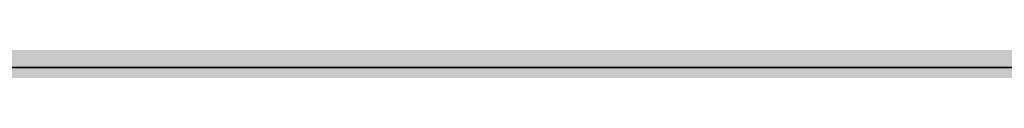
# Model space of a CAD drawing. Units: millimetres. Extents: x -22994 to 29398, y -19990 to 20176.
# Tile 96 of 135: x 229.428 to 230.597, y 84.556 to 84.571. Entities that reach past the tile are written whole.
import ezdxf
from ezdxf import colors
from ezdxf.entities.mleader import LeaderData, LeaderLine
from ezdxf.math import Vec2, Vec3

# ---------------------------------------------------------------- set-up
doc = ezdxf.new("R2010")
doc.units = ezdxf.units.MM
doc.header["$MEASUREMENT"] = 0
for name, color, linetype, lineweight in [('M-ANNO-TEXT', 7, 'Continuous', 25), ('M-DIMS', 2, 'Continuous', 18), ('M-EQPM-PATT', 7, 'Continuous', 18), ('M-PIPE', 7, 'Continuous', 35)]:
    doc.layers.add(name, color=color, linetype=linetype, lineweight=lineweight)
doc.styles.get("Standard").update_dxf_attribs({"font": 'arial.ttf'})
doc.dimstyles.get("Standard").update_dxf_attribs({"dimtxt": 0.18, "dimasz": 10000, "dimexe": 0.18, "dimexo": 0.0625, "dimgap": 0.09, "dimtad": 0, "dimtih": 1, "dimtoh": 1, "dimdec": 0, "dimzin": 0, "dimdsep": 46, "dimtxsty": 'Standard', "dimcen": 0.09, "dimadec": 0, "dimazin": 0, "dimtfac": 1, "dimtdec": 0, "dimtofl": 0, "dimtmove": 0, "dimatfit": 3, "dimfxl": 1, "dimtolj": 1, "dimtzin": 0, "dimlwd": 30, "dimarcsym": 0})

# ---------------------------------------------------------------- blocks, each defined once
blk = doc.blocks.new('*D2')
at = {"layer": 'Defpoints', "color": 0, "transparency": 16777216}
for p in [(6.6773, 10.2713), (290.852, 10.2713), (290.852, -5.0787)]:
    blk.add_point(p, dxfattribs=at)
at = {"layer": 'M-DIMS', "color": 0, "lineweight": -2, "transparency": 16777216}
for p, q in [((6.6773, 10.2088), (6.6773, -5.2587)), ((290.852, 10.2088), (290.852, -5.2587))]:
    blk.add_line(p, q, dxfattribs=at)
at = {"layer": 'M-DIMS', "color": 0, "lineweight": 30, "transparency": 16777216}
for p, q in [((-9993.3227, -5.0787), (-19993.3227, -5.0787)), ((10290.852, -5.0787), (20290.852, -5.0787))]:
    blk.add_line(p, q, dxfattribs=at)
at = {"layer": 'M-DIMS', "color": 0, "transparency": 16777216}
for points in [[(-9993.3227, 1661.5879), (-9993.3227, -1671.7454), (6.6773, -5.0787)], [(10290.852, 1661.5879), (10290.852, -1671.7454), (290.852, -5.0787)]]:
    blk.add_solid(points, dxfattribs=at)
at = {"layer": 'M-DIMS', "color": 0, "transparency": 16777216, "insert": (148.7647, -5.0787), "char_height": 0.18, "attachment_point": 5}
blk.add_mtext('\\A1;284.2', dxfattribs=at)
blk = doc.blocks.new('*D3')
at = {"layer": 'Defpoints', "color": 0, "transparency": 16777216}
for p in [(110.2647, 204.1654), (110.2647, 176.3662), (95.8327, 127.967)]:
    blk.add_point(p, dxfattribs=at)
at = {"layer": 'M-DIMS', "color": 0, "lineweight": -2, "transparency": 16777216}
for p, q in [((95.8327, 128.0295), (95.8327, 204.3454)), ((110.2647, 176.4287), (110.2647, 204.3454))]:
    blk.add_line(p, q, dxfattribs=at)
at = {"layer": 'M-DIMS', "color": 0, "lineweight": 30, "transparency": 16777216}
for p, q in [((-9904.1673, 204.1654), (-19904.1673, 204.1654)), ((10110.2647, 204.1654), (20110.2647, 204.1654))]:
    blk.add_line(p, q, dxfattribs=at)
at = {"layer": 'M-DIMS', "color": 0, "transparency": 16777216}
for points in [[(-9904.1673, 1870.8321), (-9904.1673, -1462.5013), (95.8327, 204.1654)], [(10110.2647, 1870.8321), (10110.2647, -1462.5013), (110.2647, 204.1654)]]:
    blk.add_solid(points, dxfattribs=at)
at = {"layer": 'M-DIMS', "color": 0, "transparency": 16777216, "insert": (103.0487, 204.1654), "char_height": 0.18, "attachment_point": 5}
blk.add_mtext('\\A1;14.432', dxfattribs=at)
blk = doc.blocks.new('*D4')
at = {"layer": 'Defpoints', "color": 0, "transparency": 16777216}
for p in [(116.2647, 204.1654), (110.2647, 176.3662), (116.2647, 176.3662)]:
    blk.add_point(p, dxfattribs=at)
at = {"layer": 'M-DIMS', "color": 0, "lineweight": -2, "transparency": 16777216}
for p, q in [((110.2647, 176.4287), (110.2647, 204.3454)), ((116.2647, 176.4287), (116.2647, 204.3454))]:
    blk.add_line(p, q, dxfattribs=at)
at = {"layer": 'M-DIMS', "color": 0, "lineweight": 30, "transparency": 16777216}
for p, q in [((-9889.7353, 204.1654), (-19889.7353, 204.1654)), ((10116.2647, 204.1654), (20116.2647, 204.1654))]:
    blk.add_line(p, q, dxfattribs=at)
at = {"layer": 'M-DIMS', "color": 0, "transparency": 16777216}
for points in [[(-9889.7353, 1870.8321), (-9889.7353, -1462.5013), (110.2647, 204.1654)], [(10116.2647, 1870.8321), (10116.2647, -1462.5013), (116.2647, 204.1654)]]:
    blk.add_solid(points, dxfattribs=at)
at = {"layer": 'M-DIMS', "color": 0, "transparency": 16777216, "insert": (113.2647, 204.1654), "char_height": 0.18, "attachment_point": 5}
blk.add_mtext('\\A1;6', dxfattribs=at)
blk = doc.blocks.new('*D5')
at = {"layer": 'Defpoints', "color": 0, "transparency": 16777216}
for p in [(181.2647, 204.1654), (116.2647, 176.3662), (181.2647, 176.3662)]:
    blk.add_point(p, dxfattribs=at)
at = {"layer": 'M-DIMS', "color": 0, "lineweight": -2, "transparency": 16777216}
for p, q in [((116.2647, 176.4287), (116.2647, 204.3454)), ((181.2647, 176.4287), (181.2647, 204.3454))]:
    blk.add_line(p, q, dxfattribs=at)
at = {"layer": 'M-DIMS', "color": 0, "lineweight": 30, "transparency": 16777216}
for p, q in [((-9883.7353, 204.1654), (-19883.7353, 204.1654)), ((10181.2647, 204.1654), (20181.2647, 204.1654))]:
    blk.add_line(p, q, dxfattribs=at)
at = {"layer": 'M-DIMS', "color": 0, "transparency": 16777216}
for points in [[(-9883.7353, 1870.8321), (-9883.7353, -1462.5013), (116.2647, 204.1654)], [(10181.2647, 1870.8321), (10181.2647, -1462.5013), (181.2647, 204.1654)]]:
    blk.add_solid(points, dxfattribs=at)
at = {"layer": 'M-DIMS', "color": 0, "transparency": 16777216, "insert": (148.7647, 204.1654), "char_height": 0.18, "attachment_point": 5}
blk.add_mtext('\\A1;65', dxfattribs=at)
blk = doc.blocks.new('*D6')
at = {"layer": 'Defpoints', "color": 0, "transparency": 16777216}
for p in [(187.2647, 204.1654), (181.2647, 176.3662), (187.2647, 176.3662)]:
    blk.add_point(p, dxfattribs=at)
at = {"layer": 'M-DIMS', "color": 0, "lineweight": -2, "transparency": 16777216}
for p, q in [((181.2647, 176.4287), (181.2647, 204.3454)), ((187.2647, 176.4287), (187.2647, 204.3454))]:
    blk.add_line(p, q, dxfattribs=at)
at = {"layer": 'M-DIMS', "color": 0, "lineweight": 30, "transparency": 16777216}
for p, q in [((-9818.7353, 204.1654), (-19818.7353, 204.1654)), ((10187.2647, 204.1654), (20187.2647, 204.1654))]:
    blk.add_line(p, q, dxfattribs=at)
at = {"layer": 'M-DIMS', "color": 0, "transparency": 16777216}
for points in [[(-9818.7353, 1870.8321), (-9818.7353, -1462.5013), (181.2647, 204.1654)], [(10187.2647, 1870.8321), (10187.2647, -1462.5013), (187.2647, 204.1654)]]:
    blk.add_solid(points, dxfattribs=at)
at = {"layer": 'M-DIMS', "color": 0, "transparency": 16777216, "insert": (184.2647, 204.1654), "char_height": 0.18, "attachment_point": 5}
blk.add_mtext('\\A1;6', dxfattribs=at)
blk = doc.blocks.new('*D7')
at = {"layer": 'Defpoints', "color": 0, "transparency": 16777216}
for p in [(201.6967, 204.1654), (187.2647, 176.3662), (201.6967, 127.967)]:
    blk.add_point(p, dxfattribs=at)
at = {"layer": 'M-DIMS', "color": 0, "lineweight": -2, "transparency": 16777216}
for p, q in [((187.2647, 176.4287), (187.2647, 204.3454)), ((201.6967, 128.0295), (201.6967, 204.3454))]:
    blk.add_line(p, q, dxfattribs=at)
at = {"layer": 'M-DIMS', "color": 0, "lineweight": 30, "transparency": 16777216}
for p, q in [((-9812.7353, 204.1654), (-19812.7353, 204.1654)), ((10201.6967, 204.1654), (20201.6967, 204.1654))]:
    blk.add_line(p, q, dxfattribs=at)
at = {"layer": 'M-DIMS', "color": 0, "transparency": 16777216}
for points in [[(-9812.7353, 1870.8321), (-9812.7353, -1462.5013), (187.2647, 204.1654)], [(10201.6967, 1870.8321), (10201.6967, -1462.5013), (201.6967, 204.1654)]]:
    blk.add_solid(points, dxfattribs=at)
at = {"layer": 'M-DIMS', "color": 0, "transparency": 16777216, "insert": (194.4807, 204.1654), "char_height": 0.18, "attachment_point": 5}
blk.add_mtext('\\A1;14.432', dxfattribs=at)
blk = doc.blocks.new('*D8')
at = {"layer": 'Defpoints', "color": 0, "transparency": 16777216}
for p in [(227.6485, 204.1654), (227.6485, 146.7296), (201.6967, 127.967)]:
    blk.add_point(p, dxfattribs=at)
at = {"layer": 'M-DIMS', "color": 0, "lineweight": -2, "transparency": 16777216}
for p, q in [((201.6967, 128.0295), (201.6967, 204.3454)), ((227.6485, 146.7921), (227.6485, 204.3454))]:
    blk.add_line(p, q, dxfattribs=at)
at = {"layer": 'M-DIMS', "color": 0, "lineweight": 30, "transparency": 16777216}
for p, q in [((-9798.3033, 204.1654), (-19798.3033, 204.1654)), ((10227.6485, 204.1654), (20227.6485, 204.1654))]:
    blk.add_line(p, q, dxfattribs=at)
at = {"layer": 'M-DIMS', "color": 0, "transparency": 16777216}
for points in [[(-9798.3033, 1870.8321), (-9798.3033, -1462.5013), (201.6967, 204.1654)], [(10227.6485, 1870.8321), (10227.6485, -1462.5013), (227.6485, 204.1654)]]:
    blk.add_solid(points, dxfattribs=at)
at = {"layer": 'M-DIMS', "color": 0, "transparency": 16777216, "insert": (214.6726, 204.1654), "char_height": 0.18, "attachment_point": 5}
blk.add_mtext('\\A1;25.95', dxfattribs=at)
blk = doc.blocks.new('*D9')
at = {"layer": 'Defpoints', "color": 0, "transparency": 16777216}
for p in [(187.2647, 176.3662), (306.202, 176.3662), (290.852, 10.2713)]:
    blk.add_point(p, dxfattribs=at)
at = {"layer": 'M-DIMS', "color": 0, "lineweight": 30, "transparency": 16777216}
for p, q in [((306.202, 10176.3662), (306.202, 20176.3662)), ((306.202, -9989.7287), (306.202, -19989.7287))]:
    blk.add_line(p, q, dxfattribs=at)
at = {"layer": 'M-DIMS', "color": 0, "lineweight": -2, "transparency": 16777216}
for p, q in [((187.3272, 176.3662), (306.382, 176.3662)), ((290.9145, 10.2713), (306.382, 10.2713))]:
    blk.add_line(p, q, dxfattribs=at)
at = {"layer": 'M-DIMS', "color": 0, "transparency": 16777216}
for points in [[(-1360.4646, 10176.3662), (1972.8687, 10176.3662), (306.202, 176.3662)], [(-1360.4646, -9989.7287), (1972.8687, -9989.7287), (306.202, 10.2713)]]:
    blk.add_solid(points, dxfattribs=at)
at = {"layer": 'M-DIMS', "color": 0, "transparency": 16777216, "insert": (306.202, 93.3187), "char_height": 0.18, "attachment_point": 5}
blk.add_mtext('\\A1;166.1', dxfattribs=at)
blk = doc.blocks.new('*D10')
at = {"layer": 'Defpoints', "color": 0, "transparency": 16777216}
for p in [(125.6498, 136.0713), (133.3459, 136.0713), (133.3459, -5.0787)]:
    blk.add_point(p, dxfattribs=at)
at = {"layer": 'M-DIMS', "color": 0, "lineweight": -2, "transparency": 16777216}
for p, q in [((125.6498, 136.0088), (125.6498, -5.2587)), ((133.3459, 136.0088), (133.3459, -5.2587))]:
    blk.add_line(p, q, dxfattribs=at)
at = {"layer": 'M-DIMS', "color": 0, "lineweight": 30, "transparency": 16777216}
for p, q in [((-9874.3502, -5.0787), (-19874.3502, -5.0787)), ((10133.3459, -5.0787), (20133.3459, -5.0787))]:
    blk.add_line(p, q, dxfattribs=at)
at = {"layer": 'M-DIMS', "color": 0, "transparency": 16777216}
for points in [[(-9874.3502, 1661.5879), (-9874.3502, -1671.7454), (125.6498, -5.0787)], [(10133.3459, 1661.5879), (10133.3459, -1671.7454), (133.3459, -5.0787)]]:
    blk.add_solid(points, dxfattribs=at)
at = {"layer": 'M-DIMS', "color": 0, "transparency": 16777216, "insert": (129.4978, -5.0787), "char_height": 0.18, "attachment_point": 5}
blk.add_mtext('\\A1;7.696', dxfattribs=at)
blk = doc.blocks.new('*D11')
at = {"layer": 'Defpoints', "color": 0, "transparency": 16777216}
for p in [(133.3459, 136.0713), (135.6498, 136.0713), (135.6498, -5.0787)]:
    blk.add_point(p, dxfattribs=at)
at = {"layer": 'M-DIMS', "color": 0, "lineweight": -2, "transparency": 16777216}
for p, q in [((133.3459, 136.0088), (133.3459, -5.2587)), ((135.6498, 136.0088), (135.6498, -5.2587))]:
    blk.add_line(p, q, dxfattribs=at)
at = {"layer": 'M-DIMS', "color": 0, "lineweight": 30, "transparency": 16777216}
for p, q in [((-9866.6541, -5.0787), (-19866.6541, -5.0787)), ((10135.6498, -5.0787), (20135.6498, -5.0787))]:
    blk.add_line(p, q, dxfattribs=at)
at = {"layer": 'M-DIMS', "color": 0, "transparency": 16777216}
for points in [[(-9866.6541, 1661.5879), (-9866.6541, -1671.7454), (133.3459, -5.0787)], [(10135.6498, 1661.5879), (10135.6498, -1671.7454), (135.6498, -5.0787)]]:
    blk.add_solid(points, dxfattribs=at)
at = {"layer": 'M-DIMS', "color": 0, "transparency": 16777216, "insert": (134.4978, -5.0787), "char_height": 0.18, "attachment_point": 5}
blk.add_mtext('\\A1;2.304', dxfattribs=at)
blk = doc.blocks.new('*D12')
at = {"layer": 'Defpoints', "color": 0, "transparency": 16777216}
for p in [(135.6498, 136.0713), (145.6498, 136.0713), (145.6498, -5.0787)]:
    blk.add_point(p, dxfattribs=at)
at = {"layer": 'M-DIMS', "color": 0, "lineweight": -2, "transparency": 16777216}
for p, q in [((135.6498, 136.0088), (135.6498, -5.2587)), ((145.6498, 136.0088), (145.6498, -5.2587))]:
    blk.add_line(p, q, dxfattribs=at)
at = {"layer": 'M-DIMS', "color": 0, "lineweight": 30, "transparency": 16777216}
for p, q in [((-9864.3502, -5.0787), (-19864.3502, -5.0787)), ((10145.6498, -5.0787), (20145.6498, -5.0787))]:
    blk.add_line(p, q, dxfattribs=at)
at = {"layer": 'M-DIMS', "color": 0, "transparency": 16777216}
for points in [[(-9864.3502, 1661.5879), (-9864.3502, -1671.7454), (135.6498, -5.0787)], [(10145.6498, 1661.5879), (10145.6498, -1671.7454), (145.6498, -5.0787)]]:
    blk.add_solid(points, dxfattribs=at)
at = {"layer": 'M-DIMS', "color": 0, "transparency": 16777216, "insert": (140.6498, -5.0787), "char_height": 0.18, "attachment_point": 5}
blk.add_mtext('\\A1;10', dxfattribs=at)
blk = doc.blocks.new('*D13')
at = {"layer": 'Defpoints', "color": 0, "transparency": 16777216}
for p in [(145.6498, 136.0713), (155.6498, 136.0713), (155.6498, -5.0787)]:
    blk.add_point(p, dxfattribs=at)
at = {"layer": 'M-DIMS', "color": 0, "lineweight": -2, "transparency": 16777216}
for p, q in [((145.6498, 136.0088), (145.6498, -5.2587)), ((155.6498, 136.0088), (155.6498, -5.2587))]:
    blk.add_line(p, q, dxfattribs=at)
at = {"layer": 'M-DIMS', "color": 0, "lineweight": 30, "transparency": 16777216}
for p, q in [((-9854.3502, -5.0787), (-19854.3502, -5.0787)), ((10155.6498, -5.0787), (20155.6498, -5.0787))]:
    blk.add_line(p, q, dxfattribs=at)
at = {"layer": 'M-DIMS', "color": 0, "transparency": 16777216}
for points in [[(-9854.3502, 1661.5879), (-9854.3502, -1671.7454), (145.6498, -5.0787)], [(10155.6498, 1661.5879), (10155.6498, -1671.7454), (155.6498, -5.0787)]]:
    blk.add_solid(points, dxfattribs=at)
at = {"layer": 'M-DIMS', "color": 0, "transparency": 16777216, "insert": (150.6498, -5.0787), "char_height": 0.18, "attachment_point": 5}
blk.add_mtext('\\A1;10', dxfattribs=at)
blk = doc.blocks.new('*D14')
at = {"layer": 'Defpoints', "color": 0, "transparency": 16777216}
for p in [(155.6498, 136.0713), (165.6498, 136.0713), (165.6498, -5.0787)]:
    blk.add_point(p, dxfattribs=at)
at = {"layer": 'M-DIMS', "color": 0, "lineweight": -2, "transparency": 16777216}
for p, q in [((155.6498, 136.0088), (155.6498, -5.2587)), ((165.6498, 136.0088), (165.6498, -5.2587))]:
    blk.add_line(p, q, dxfattribs=at)
at = {"layer": 'M-DIMS', "color": 0, "lineweight": 30, "transparency": 16777216}
for p, q in [((-9844.3502, -5.0787), (-19844.3502, -5.0787)), ((10165.6498, -5.0787), (20165.6498, -5.0787))]:
    blk.add_line(p, q, dxfattribs=at)
at = {"layer": 'M-DIMS', "color": 0, "transparency": 16777216}
for points in [[(-9844.3502, 1661.5879), (-9844.3502, -1671.7454), (155.6498, -5.0787)], [(10165.6498, 1661.5879), (10165.6498, -1671.7454), (165.6498, -5.0787)]]:
    blk.add_solid(points, dxfattribs=at)
at = {"layer": 'M-DIMS', "color": 0, "transparency": 16777216, "insert": (160.6498, -5.0787), "char_height": 0.18, "attachment_point": 5}
blk.add_mtext('\\A1;10', dxfattribs=at)
blk = doc.blocks.new('*D15')
at = {"layer": 'Defpoints', "color": 0, "transparency": 16777216}
for p in [(173.3459, 154.788), (173.3459, 136.0713), (306.202, 136.0713)]:
    blk.add_point(p, dxfattribs=at)
at = {"layer": 'M-DIMS', "color": 0, "lineweight": 30, "transparency": 16777216}
for p, q in [((306.202, 10154.788), (306.202, 20154.788)), ((306.202, -9863.9287), (306.202, -19863.9287))]:
    blk.add_line(p, q, dxfattribs=at)
at = {"layer": 'M-DIMS', "color": 0, "lineweight": -2, "transparency": 16777216}
for p, q in [((173.4084, 154.788), (306.382, 154.788)), ((173.4084, 136.0713), (306.382, 136.0713))]:
    blk.add_line(p, q, dxfattribs=at)
at = {"layer": 'M-DIMS', "color": 0, "transparency": 16777216}
for points in [[(-1360.4646, 10154.788), (1972.8687, 10154.788), (306.202, 154.788)], [(-1360.4646, -9863.9287), (1972.8687, -9863.9287), (306.202, 136.0713)]]:
    blk.add_solid(points, dxfattribs=at)
at = {"layer": 'M-DIMS', "color": 0, "transparency": 16777216, "insert": (306.202, 145.4297), "char_height": 0.18, "attachment_point": 5}
blk.add_mtext('\\A1;18.717', dxfattribs=at)
blk = doc.blocks.new('*D16')
at = {"layer": 'Defpoints', "color": 0, "transparency": 16777216}
for p in [(120.1702, 204.1654), (110.4658, 48.0349), (120.1702, 48.0349)]:
    blk.add_point(p, dxfattribs=at)
at = {"layer": 'M-DIMS', "color": 0, "lineweight": -2, "transparency": 16777216}
for p, q in [((110.4658, 48.0974), (110.4658, 204.3454)), ((120.1702, 48.0974), (120.1702, 204.3454))]:
    blk.add_line(p, q, dxfattribs=at)
at = {"layer": 'M-DIMS', "color": 0, "lineweight": 30, "transparency": 16777216}
for p, q in [((-9889.5342, 204.1654), (-19889.5342, 204.1654)), ((10120.1702, 204.1654), (20120.1702, 204.1654))]:
    blk.add_line(p, q, dxfattribs=at)
at = {"layer": 'M-DIMS', "color": 0, "transparency": 16777216}
for points in [[(-9889.5342, 1870.8321), (-9889.5342, -1462.5013), (110.4658, 204.1654)], [(10120.1702, 1870.8321), (10120.1702, -1462.5013), (120.1702, 204.1654)]]:
    blk.add_solid(points, dxfattribs=at)
at = {"layer": 'M-DIMS', "color": 0, "transparency": 16777216, "insert": (115.318, 204.1654), "char_height": 0.18, "attachment_point": 5}
blk.add_mtext('\\A1;9.704', dxfattribs=at)
blk = doc.blocks.new('*D17')
at = {"layer": 'Defpoints', "color": 0, "transparency": 16777216}
for p in [(126.1702, 204.1654), (120.1702, 48.0349), (126.1702, 48.0349)]:
    blk.add_point(p, dxfattribs=at)
at = {"layer": 'M-DIMS', "color": 0, "lineweight": -2, "transparency": 16777216}
for p, q in [((120.1702, 48.0974), (120.1702, 204.3454)), ((126.1702, 48.0974), (126.1702, 204.3454))]:
    blk.add_line(p, q, dxfattribs=at)
at = {"layer": 'M-DIMS', "color": 0, "lineweight": 30, "transparency": 16777216}
for p, q in [((-9879.8298, 204.1654), (-19879.8298, 204.1654)), ((10126.1702, 204.1654), (20126.1702, 204.1654))]:
    blk.add_line(p, q, dxfattribs=at)
at = {"layer": 'M-DIMS', "color": 0, "transparency": 16777216}
for points in [[(-9879.8298, 1870.8321), (-9879.8298, -1462.5013), (120.1702, 204.1654)], [(10126.1702, 1870.8321), (10126.1702, -1462.5013), (126.1702, 204.1654)]]:
    blk.add_solid(points, dxfattribs=at)
at = {"layer": 'M-DIMS', "color": 0, "transparency": 16777216, "insert": (123.1702, 204.1654), "char_height": 0.18, "attachment_point": 5}
blk.add_mtext('\\A1;6', dxfattribs=at)
blk = doc.blocks.new('*D18')
at = {"layer": 'Defpoints', "color": 0, "transparency": 16777216}
for p in [(132.1702, 204.1654), (126.1702, 48.0349), (132.1702, 48.0349)]:
    blk.add_point(p, dxfattribs=at)
at = {"layer": 'M-DIMS', "color": 0, "lineweight": -2, "transparency": 16777216}
for p, q in [((126.1702, 48.0974), (126.1702, 204.3454)), ((132.1702, 48.0974), (132.1702, 204.3454))]:
    blk.add_line(p, q, dxfattribs=at)
at = {"layer": 'M-DIMS', "color": 0, "lineweight": 30, "transparency": 16777216}
for p, q in [((-9873.8298, 204.1654), (-19873.8298, 204.1654)), ((10132.1702, 204.1654), (20132.1702, 204.1654))]:
    blk.add_line(p, q, dxfattribs=at)
at = {"layer": 'M-DIMS', "color": 0, "transparency": 16777216}
for points in [[(-9873.8298, 1870.8321), (-9873.8298, -1462.5013), (126.1702, 204.1654)], [(10132.1702, 1870.8321), (10132.1702, -1462.5013), (132.1702, 204.1654)]]:
    blk.add_solid(points, dxfattribs=at)
at = {"layer": 'M-DIMS', "color": 0, "transparency": 16777216, "insert": (129.1702, 204.1654), "char_height": 0.18, "attachment_point": 5}
blk.add_mtext('\\A1;6', dxfattribs=at)
blk = doc.blocks.new('*D19')
at = {"layer": 'Defpoints', "color": 0, "transparency": 16777216}
for p in [(138.1702, 204.1654), (132.1702, 48.0349), (138.1702, 48.0349)]:
    blk.add_point(p, dxfattribs=at)
at = {"layer": 'M-DIMS', "color": 0, "lineweight": -2, "transparency": 16777216}
for p, q in [((132.1702, 48.0974), (132.1702, 204.3454)), ((138.1702, 48.0974), (138.1702, 204.3454))]:
    blk.add_line(p, q, dxfattribs=at)
at = {"layer": 'M-DIMS', "color": 0, "lineweight": 30, "transparency": 16777216}
for p, q in [((-9867.8298, 204.1654), (-19867.8298, 204.1654)), ((10138.1702, 204.1654), (20138.1702, 204.1654))]:
    blk.add_line(p, q, dxfattribs=at)
at = {"layer": 'M-DIMS', "color": 0, "transparency": 16777216}
for points in [[(-9867.8298, 1870.8321), (-9867.8298, -1462.5013), (132.1702, 204.1654)], [(10138.1702, 1870.8321), (10138.1702, -1462.5013), (138.1702, 204.1654)]]:
    blk.add_solid(points, dxfattribs=at)
at = {"layer": 'M-DIMS', "color": 0, "transparency": 16777216, "insert": (135.1702, 204.1654), "char_height": 0.18, "attachment_point": 5}
blk.add_mtext('\\A1;6', dxfattribs=at)
blk = doc.blocks.new('*D20')
at = {"layer": 'Defpoints', "color": 0, "transparency": 16777216}
for p in [(144.1702, 204.1654), (138.1702, 48.0349), (144.1702, 48.0349)]:
    blk.add_point(p, dxfattribs=at)
at = {"layer": 'M-DIMS', "color": 0, "lineweight": -2, "transparency": 16777216}
for p, q in [((138.1702, 48.0974), (138.1702, 204.3454)), ((144.1702, 48.0974), (144.1702, 204.3454))]:
    blk.add_line(p, q, dxfattribs=at)
at = {"layer": 'M-DIMS', "color": 0, "lineweight": 30, "transparency": 16777216}
for p, q in [((-9861.8298, 204.1654), (-19861.8298, 204.1654)), ((10144.1702, 204.1654), (20144.1702, 204.1654))]:
    blk.add_line(p, q, dxfattribs=at)
at = {"layer": 'M-DIMS', "color": 0, "transparency": 16777216}
for points in [[(-9861.8298, 1870.8321), (-9861.8298, -1462.5013), (138.1702, 204.1654)], [(10144.1702, 1870.8321), (10144.1702, -1462.5013), (144.1702, 204.1654)]]:
    blk.add_solid(points, dxfattribs=at)
at = {"layer": 'M-DIMS', "color": 0, "transparency": 16777216, "insert": (141.1702, 204.1654), "char_height": 0.18, "attachment_point": 5}
blk.add_mtext('\\A1;6', dxfattribs=at)
blk = doc.blocks.new('*D21')
at = {"layer": 'Defpoints', "color": 0, "transparency": 16777216}
for p in [(149.1157, 204.1654), (144.1702, 48.0349), (149.1157, 48.0349)]:
    blk.add_point(p, dxfattribs=at)
at = {"layer": 'M-DIMS', "color": 0, "lineweight": -2, "transparency": 16777216}
for p, q in [((144.1702, 48.0974), (144.1702, 204.3454)), ((149.1157, 48.0974), (149.1157, 204.3454))]:
    blk.add_line(p, q, dxfattribs=at)
at = {"layer": 'M-DIMS', "color": 0, "lineweight": 30, "transparency": 16777216}
for p, q in [((-9855.8298, 204.1654), (-19855.8298, 204.1654)), ((10149.1157, 204.1654), (20149.1157, 204.1654))]:
    blk.add_line(p, q, dxfattribs=at)
at = {"layer": 'M-DIMS', "color": 0, "transparency": 16777216}
for points in [[(-9855.8298, 1870.8321), (-9855.8298, -1462.5013), (144.1702, 204.1654)], [(10149.1157, 1870.8321), (10149.1157, -1462.5013), (149.1157, 204.1654)]]:
    blk.add_solid(points, dxfattribs=at)
at = {"layer": 'M-DIMS', "color": 0, "transparency": 16777216, "insert": (146.6429, 204.1654), "char_height": 0.18, "attachment_point": 5}
blk.add_mtext('\\A1;4.945', dxfattribs=at)
blk = doc.blocks.new('*D22')
at = {"layer": 'Defpoints', "color": 0, "transparency": 16777216}
for p in [(149.1157, 30.9895), (155.1157, 30.9895), (155.1157, -5.0787)]:
    blk.add_point(p, dxfattribs=at)
at = {"layer": 'M-DIMS', "color": 0, "lineweight": -2, "transparency": 16777216}
for p, q in [((149.1157, 30.927), (149.1157, -5.2587)), ((155.1157, 30.927), (155.1157, -5.2587))]:
    blk.add_line(p, q, dxfattribs=at)
at = {"layer": 'M-DIMS', "color": 0, "lineweight": 30, "transparency": 16777216}
for p, q in [((-9850.8843, -5.0787), (-19850.8843, -5.0787)), ((10155.1157, -5.0787), (20155.1157, -5.0787))]:
    blk.add_line(p, q, dxfattribs=at)
at = {"layer": 'M-DIMS', "color": 0, "transparency": 16777216}
for points in [[(-9850.8843, 1661.5879), (-9850.8843, -1671.7454), (149.1157, -5.0787)], [(10155.1157, 1661.5879), (10155.1157, -1671.7454), (155.1157, -5.0787)]]:
    blk.add_solid(points, dxfattribs=at)
at = {"layer": 'M-DIMS', "color": 0, "transparency": 16777216, "insert": (152.1157, -5.0787), "char_height": 0.18, "attachment_point": 5}
blk.add_mtext('\\A1;6', dxfattribs=at)
blk = doc.blocks.new('*D23')
at = {"layer": 'Defpoints', "color": 0, "transparency": 16777216}
for p in [(155.1157, 30.9895), (161.1157, 30.9895), (161.1157, -5.0787)]:
    blk.add_point(p, dxfattribs=at)
at = {"layer": 'M-DIMS', "color": 0, "lineweight": -2, "transparency": 16777216}
for p, q in [((155.1157, 30.927), (155.1157, -5.2587)), ((161.1157, 30.927), (161.1157, -5.2587))]:
    blk.add_line(p, q, dxfattribs=at)
at = {"layer": 'M-DIMS', "color": 0, "lineweight": 30, "transparency": 16777216}
for p, q in [((-9844.8843, -5.0787), (-19844.8843, -5.0787)), ((10161.1157, -5.0787), (20161.1157, -5.0787))]:
    blk.add_line(p, q, dxfattribs=at)
at = {"layer": 'M-DIMS', "color": 0, "transparency": 16777216}
for points in [[(-9844.8843, 1661.5879), (-9844.8843, -1671.7454), (155.1157, -5.0787)], [(10161.1157, 1661.5879), (10161.1157, -1671.7454), (161.1157, -5.0787)]]:
    blk.add_solid(points, dxfattribs=at)
at = {"layer": 'M-DIMS', "color": 0, "transparency": 16777216, "insert": (158.1157, -5.0787), "char_height": 0.18, "attachment_point": 5}
blk.add_mtext('\\A1;6', dxfattribs=at)
blk = doc.blocks.new('*D24')
at = {"layer": 'Defpoints', "color": 0, "transparency": 16777216}
for p in [(161.1157, 30.9895), (166.4387, 30.9895), (166.4387, -5.0787)]:
    blk.add_point(p, dxfattribs=at)
at = {"layer": 'M-DIMS', "color": 0, "lineweight": -2, "transparency": 16777216}
for p, q in [((161.1157, 30.927), (161.1157, -5.2587)), ((166.4387, 30.927), (166.4387, -5.2587))]:
    blk.add_line(p, q, dxfattribs=at)
at = {"layer": 'M-DIMS', "color": 0, "lineweight": 30, "transparency": 16777216}
for p, q in [((-9838.8843, -5.0787), (-19838.8843, -5.0787)), ((10166.4387, -5.0787), (20166.4387, -5.0787))]:
    blk.add_line(p, q, dxfattribs=at)
at = {"layer": 'M-DIMS', "color": 0, "transparency": 16777216}
for points in [[(-9838.8843, 1661.5879), (-9838.8843, -1671.7454), (161.1157, -5.0787)], [(10166.4387, 1661.5879), (10166.4387, -1671.7454), (166.4387, -5.0787)]]:
    blk.add_solid(points, dxfattribs=at)
at = {"layer": 'M-DIMS', "color": 0, "transparency": 16777216, "insert": (163.7772, -5.0787), "char_height": 0.18, "attachment_point": 5}
blk.add_mtext('\\A1;5.323', dxfattribs=at)
blk = doc.blocks.new('*D25')
at = {"layer": 'Defpoints', "color": 0, "transparency": 16777216}
for p in [(166.4387, 30.9895), (172.4387, 30.9895), (172.4387, -5.0787)]:
    blk.add_point(p, dxfattribs=at)
at = {"layer": 'M-DIMS', "color": 0, "lineweight": -2, "transparency": 16777216}
for p, q in [((166.4387, 30.927), (166.4387, -5.2587)), ((172.4387, 30.927), (172.4387, -5.2587))]:
    blk.add_line(p, q, dxfattribs=at)
at = {"layer": 'M-DIMS', "color": 0, "lineweight": 30, "transparency": 16777216}
for p, q in [((-9833.5613, -5.0787), (-19833.5613, -5.0787)), ((10172.4387, -5.0787), (20172.4387, -5.0787))]:
    blk.add_line(p, q, dxfattribs=at)
at = {"layer": 'M-DIMS', "color": 0, "transparency": 16777216}
for points in [[(-9833.5613, 1661.5879), (-9833.5613, -1671.7454), (166.4387, -5.0787)], [(10172.4387, 1661.5879), (10172.4387, -1671.7454), (172.4387, -5.0787)]]:
    blk.add_solid(points, dxfattribs=at)
at = {"layer": 'M-DIMS', "color": 0, "transparency": 16777216, "insert": (169.4387, -5.0787), "char_height": 0.18, "attachment_point": 5}
blk.add_mtext('\\A1;6', dxfattribs=at)
blk = doc.blocks.new('*D26')
at = {"layer": 'Defpoints', "color": 0, "transparency": 16777216}
for p in [(172.4387, 30.9895), (178.4387, 30.9895), (178.4387, -5.0787)]:
    blk.add_point(p, dxfattribs=at)
at = {"layer": 'M-DIMS', "color": 0, "lineweight": -2, "transparency": 16777216}
for p, q in [((172.4387, 30.927), (172.4387, -5.2587)), ((178.4387, 30.927), (178.4387, -5.2587))]:
    blk.add_line(p, q, dxfattribs=at)
at = {"layer": 'M-DIMS', "color": 0, "lineweight": 30, "transparency": 16777216}
for p, q in [((-9827.5613, -5.0787), (-19827.5613, -5.0787)), ((10178.4387, -5.0787), (20178.4387, -5.0787))]:
    blk.add_line(p, q, dxfattribs=at)
at = {"layer": 'M-DIMS', "color": 0, "transparency": 16777216}
for points in [[(-9827.5613, 1661.5879), (-9827.5613, -1671.7454), (172.4387, -5.0787)], [(10178.4387, 1661.5879), (10178.4387, -1671.7454), (178.4387, -5.0787)]]:
    blk.add_solid(points, dxfattribs=at)
at = {"layer": 'M-DIMS', "color": 0, "transparency": 16777216, "insert": (175.4387, -5.0787), "char_height": 0.18, "attachment_point": 5}
blk.add_mtext('\\A1;6', dxfattribs=at)
blk = doc.blocks.new('*D27')
at = {"layer": 'Defpoints', "color": 0, "transparency": 16777216}
for p in [(178.4387, 30.9895), (188.1175, 30.9895), (188.1175, -5.0787)]:
    blk.add_point(p, dxfattribs=at)
at = {"layer": 'M-DIMS', "color": 0, "lineweight": -2, "transparency": 16777216}
for p, q in [((178.4387, 30.927), (178.4387, -5.2587)), ((188.1175, 30.927), (188.1175, -5.2587))]:
    blk.add_line(p, q, dxfattribs=at)
at = {"layer": 'M-DIMS', "color": 0, "lineweight": 30, "transparency": 16777216}
for p, q in [((-9821.5613, -5.0787), (-19821.5613, -5.0787)), ((10188.1175, -5.0787), (20188.1175, -5.0787))]:
    blk.add_line(p, q, dxfattribs=at)
at = {"layer": 'M-DIMS', "color": 0, "transparency": 16777216}
for points in [[(-9821.5613, 1661.5879), (-9821.5613, -1671.7454), (178.4387, -5.0787)], [(10188.1175, 1661.5879), (10188.1175, -1671.7454), (188.1175, -5.0787)]]:
    blk.add_solid(points, dxfattribs=at)
at = {"layer": 'M-DIMS', "color": 0, "transparency": 16777216, "insert": (183.2781, -5.0787), "char_height": 0.18, "attachment_point": 5}
blk.add_mtext('\\A1;9.679', dxfattribs=at)
blk = doc.blocks.new('*D28')
at = {"layer": 'Defpoints', "color": 0, "transparency": 16777216}
for p in [(188.1175, 48.0349), (306.202, 48.0349), (188.1175, 30.9895)]:
    blk.add_point(p, dxfattribs=at)
at = {"layer": 'M-DIMS', "color": 0, "lineweight": 30, "transparency": 16777216}
for p, q in [((306.202, 10048.0349), (306.202, 20048.0349)), ((306.202, -9969.0105), (306.202, -19969.0105))]:
    blk.add_line(p, q, dxfattribs=at)
at = {"layer": 'M-DIMS', "color": 0, "lineweight": -2, "transparency": 16777216}
for p, q in [((188.18, 48.0349), (306.382, 48.0349)), ((188.18, 30.9895), (306.382, 30.9895))]:
    blk.add_line(p, q, dxfattribs=at)
at = {"layer": 'M-DIMS', "color": 0, "transparency": 16777216}
for points in [[(-1360.4646, 10048.0349), (1972.8687, 10048.0349), (306.202, 48.0349)], [(-1360.4646, -9969.0105), (1972.8687, -9969.0105), (306.202, 30.9895)]]:
    blk.add_solid(points, dxfattribs=at)
at = {"layer": 'M-DIMS', "color": 0, "transparency": 16777216, "insert": (306.202, 39.5122), "char_height": 0.18, "attachment_point": 5}
blk.add_mtext('\\A1;17.045', dxfattribs=at)
blk = doc.blocks.new('*D29')
at = {"layer": 'Defpoints', "color": 0, "transparency": 16777216}
for p in [(36.8006, 80.045), (64.0296, 80.045)]:
    blk.add_point(p, dxfattribs=at)
at = {"layer": 'M-DIMS', "color": 0, "lineweight": -2, "transparency": 16777216}
for p, q in [((50.4151, 79.955), (50.4151, 80.135)), ((50.3251, 80.045), (50.5051, 80.045))]:
    blk.add_line(p, q, dxfattribs=at)
at = {"layer": 'M-DIMS', "color": 0, "lineweight": 30, "transparency": 16777216}
blk.add_line((20064.0296, 80.0303), (10064.0296, 80.0377), dxfattribs=at)
at = {"layer": 'M-DIMS', "color": 0, "transparency": 16777216}
blk.add_solid([(10064.0309, 1746.7043), (10064.0284, -1586.629), (64.0296, 80.045)], dxfattribs=at)
at = {"layer": 'M-DIMS', "color": 0, "transparency": 16777216, "insert": (20064.5213, 80.0303), "char_height": 0.18, "attachment_point": 5}
blk.add_mtext('\\A1;∅27.23', dxfattribs=at)
blk = doc.blocks.new('*D30')
at = {"layer": 'Defpoints', "color": 0, "transparency": 16777216}
for p in [(216.3148, 146.7291), (238.9821, 146.73)]:
    blk.add_point(p, dxfattribs=at)
at = {"layer": 'M-DIMS', "color": 0, "lineweight": 30, "transparency": 16777216}
blk.add_line((20238.9821, 147.4959), (10238.9821, 147.1129), dxfattribs=at)
at = {"layer": 'M-DIMS', "color": 0, "lineweight": -2, "transparency": 16777216}
for p, q in [((227.6485, 146.6396), (227.6485, 146.8196)), ((227.5585, 146.7296), (227.7385, 146.7296))]:
    blk.add_line(p, q, dxfattribs=at)
at = {"layer": 'M-DIMS', "color": 0, "transparency": 16777216}
blk.add_solid([(10238.9183, 1813.7796), (10239.0459, -1519.5537), (238.9821, 146.73)], dxfattribs=at)
at = {"layer": 'M-DIMS', "color": 0, "transparency": 16777216, "insert": (20239.5436, 147.4959), "char_height": 0.18, "attachment_point": 5}
blk.add_mtext('\\A1;∅22.667', dxfattribs=at)
blk = doc.blocks.new('*D31')
at = {"layer": 'Defpoints', "color": 0, "transparency": 16777216}
for p in [(223.1641, 146.7291), (232.1328, 146.73)]:
    blk.add_point(p, dxfattribs=at)
at = {"layer": 'M-DIMS', "color": 0, "lineweight": 30, "transparency": 16777216}
blk.add_line((20232.1327, 148.6656), (10232.1328, 147.6978), dxfattribs=at)
at = {"layer": 'M-DIMS', "color": 0, "lineweight": -2, "transparency": 16777216}
for p, q in [((227.6485, 146.6396), (227.6485, 146.8196)), ((227.5585, 146.7296), (227.7385, 146.7296))]:
    blk.add_line(p, q, dxfattribs=at)
at = {"layer": 'M-DIMS', "color": 0, "transparency": 16777216}
blk.add_solid([(10231.9715, 1814.3645), (10232.2941, -1518.9688), (232.1328, 146.73)], dxfattribs=at)
at = {"layer": 'M-DIMS', "color": 0, "transparency": 16777216, "insert": (20232.6245, 148.6656), "char_height": 0.18, "attachment_point": 5}
blk.add_mtext('\\A1;∅8.969', dxfattribs=at)
blk = doc.blocks.new('*D33')
at = {"layer": 'Defpoints', "color": 0, "transparency": 16777216}
for p in [(229.5613, 154.3773), (232.9972, 153.3509)]:
    blk.add_point(p, dxfattribs=at)
at = {"layer": 'M-DIMS', "color": 0, "lineweight": -2, "transparency": 16777216}
for p, q in [((229.5613, 154.2873), (229.5613, 154.4673)), ((229.4713, 154.3773), (229.6513, 154.3773))]:
    blk.add_line(p, q, dxfattribs=at)
at = {"layer": 'M-DIMS', "color": 0, "lineweight": 30, "transparency": 16777216}
for p, q in [((19396.3388, -5570.8378), (9814.668, -2708.7434)), ((29396.3388, -5570.8378), (19396.3388, -5570.8378))]:
    blk.add_line(p, q, dxfattribs=at)
at = {"layer": 'M-DIMS', "color": 0, "transparency": 16777216}
blk.add_solid([(10291.6837, -1111.7983), (9337.6523, -4305.6886), (232.9972, 153.3509)], dxfattribs=at)
at = {"layer": 'M-DIMS', "color": 0, "transparency": 16777216, "insert": (29397.0125, -5570.8378), "char_height": 0.18, "attachment_point": 5}
blk.add_mtext('\\A1;6X R3.586', dxfattribs=at)
blk = doc.blocks.new('*D36')
at = {"layer": 'Defpoints', "color": 0, "transparency": 16777216}
for p in [(46.39, 31.3035), (46.3875, 26.5934)]:
    blk.add_point(p, dxfattribs=at)
at = {"layer": 'M-DIMS', "color": 0, "lineweight": 30, "transparency": 16777216}
for p, q in [((57.1499, 20031.3006), (51.77, 10031.302)), ((10057.1499, 20031.3006), (57.1499, 20031.3006))]:
    blk.add_line(p, q, dxfattribs=at)
at = {"layer": 'M-DIMS', "color": 0, "lineweight": -2, "transparency": 16777216}
for p, q in [((46.3887, 28.8585), (46.3887, 29.0385)), ((46.2987, 28.9485), (46.4787, 28.9485))]:
    blk.add_line(p, q, dxfattribs=at)
at = {"layer": 'M-DIMS', "color": 0, "transparency": 16777216}
blk.add_solid([(-1614.8965, 10032.1987), (1718.4364, 10030.4054), (46.39, 31.3035)], dxfattribs=at)
at = {"layer": 'M-DIMS', "color": 0, "transparency": 16777216, "insert": (10057.5542, 20031.3006), "char_height": 0.18, "attachment_point": 5}
blk.add_mtext('\\A1;∅4.71', dxfattribs=at)

msp = doc.modelspace()

# ---------------------------------------------------------------- hatches: boundary and pattern name
at = {"layer": 'M-EQPM-PATT'}
h = msp.add_hatch(color=256, dxfattribs=at)
h.set_gradient(color1=(205, 32, 39), color2=(205, 32, 39), tint=1)
h.paths.add_polyline_path([(116.2647, 150.3662), (116.2647, 170.3662), (116.2647, 176.3662), (110.2647, 176.3662), (110.2647, 152.0276), (95.8327, 127.967), (95.8327, 16.6063), (201.6967, 16.6063), (201.6967, 127.967), (187.2647, 152.0276), (187.2647, 176.3662), (181.2647, 176.3662), (181.2647, 170.3662), (181.2647, 150.3662), (195.6967, 126.3055), (195.6967, 22.6063), (101.8327, 22.6063), (101.8327, 126.3055)])
h.paths.add_polyline_path([(185.2208, 88.6347), (101.8327, 88.6347), (101.8327, 87.6347), (182.8066, 87.6347), (178.7313, 83.5594), (195.6967, 83.5594), (195.6967, 84.5594), (181.1455, 84.5594)], flags=17)
h.paths.add_polyline_path([(95.8327, 88.6347), (60.9779, 88.6347, -0.022855), (61.7178, 87.6347), (95.8327, 87.6347)])
h.paths.add_polyline_path([(215.6212, 86.5189), (215.6212, 80.5999), (220.5095, 83.5594)])
h.paths.add_polyline_path([(215.6212, 84.5594), (201.6967, 84.5594), (201.6967, 83.5594), (215.6212, 83.5594)])
h.paths.add_polyline_path([(225.3978, 86.5189), (220.5095, 83.5594), (225.3978, 80.5999)])
h.paths.add_polyline_path([(231.6256, 84.5594), (225.3978, 84.5594), (225.3978, 83.5594), (231.6256, 83.5594)])

# ---------------------------------------------------------------- linework, layer by layer
at = {"layer": 'M-PIPE'}
msp.add_line((225.3978, 84.5594), (231.6256, 84.5594), dxfattribs=at)

# ---------------------------------------------------------------- dimensions: what is measured, and where the dimension line sits
at = {"layer": 'M-DIMS'}
for base, p1, p2, override, picture, middle in [((306.202, 176.3662), (290.852, 10.2713), (187.2647, 176.3662), {"dimdec": 1, "dimlfac": 1, "dimrnd": 0, "dimzin": 0, "dimdsep": 46, "dimlunit": 2}, '*D9', (306.202, 93.3187)), ((306.202, 136.0713), (173.3459, 154.788), (173.3459, 136.0713), {"dimdec": 3, "dimlfac": 1, "dimrnd": 0, "dimzin": 0, "dimdsep": 46, "dimlunit": 2}, '*D15', (306.202, 145.4297)), ((306.202, 48.0349), (188.1175, 30.9895), (188.1175, 48.0349), {"dimdec": 3, "dimlfac": 1, "dimrnd": 0, "dimzin": 0, "dimdsep": 46, "dimlunit": 2}, '*D28', (306.202, 39.5122))]:
    dim = msp.add_linear_dim(base=base, p1=p1, p2=p2, angle=90, dimstyle='Standard', override=override, dxfattribs=at)
    dim.commit()
    dim.dimension.update_dxf_attribs({"geometry": picture, "text_midpoint": middle})
for p1, p2, override, picture, middle in [((46.3875, 26.5934), (46.39, 31.3035), {"dimdec": 2, "dimlfac": 1, "dimrnd": 0, "dimzin": 0, "dimdsep": 46, "dimlunit": 2}, '*D36', (10057.5542, 20031.3006)), ((223.1641, 146.7291), (232.1328, 146.73), {"dimdec": 3, "dimlfac": 1, "dimrnd": 0, "dimzin": 0, "dimdsep": 46, "dimlunit": 2}, '*D31', (20232.1327, 148.6656)), ((216.3148, 146.7291), (238.9821, 146.73), {"dimdec": 3, "dimlfac": 1, "dimrnd": 0, "dimzin": 0, "dimdsep": 46, "dimlunit": 2}, '*D30', (20238.9821, 147.4959))]:
    dim = msp.add_diameter_dim_2p(p1=p1, p2=p2, dimstyle='Standard', override=override, dxfattribs=at)
    dim.commit()
    dim.dimension.update_dxf_attribs({"geometry": picture, "text_midpoint": middle, "dimtype": 163})
for base, p1, p2, override, picture, middle in [((110.2647, 204.1654), (95.8327, 127.967), (110.2647, 176.3662), {"dimdec": 3, "dimlfac": 1, "dimrnd": 0, "dimzin": 0, "dimdsep": 46, "dimlunit": 2}, '*D3', (103.0487, 204.1654)), ((116.2647, 204.1654), (110.2647, 176.3662), (116.2647, 176.3662), {"dimdec": 0, "dimlfac": 1, "dimrnd": 0, "dimzin": 0, "dimdsep": 46, "dimlunit": 2}, '*D4', (113.2647, 204.1654)), ((120.1702, 204.1654), (110.4658, 48.0349), (120.1702, 48.0349), {"dimdec": 3, "dimlfac": 1, "dimrnd": 0, "dimzin": 0, "dimdsep": 46, "dimlunit": 2}, '*D16', (115.318, 204.1654)), ((181.2647, 204.1654), (116.2647, 176.3662), (181.2647, 176.3662), {"dimdec": 0, "dimlfac": 1, "dimrnd": 0, "dimzin": 0, "dimdsep": 46, "dimlunit": 2}, '*D5', (148.7647, 204.1654)), ((126.1702, 204.1654), (120.1702, 48.0349), (126.1702, 48.0349), {"dimdec": 0, "dimlfac": 1, "dimrnd": 0, "dimzin": 0, "dimdsep": 46, "dimlunit": 2}, '*D17', (123.1702, 204.1654)), ((132.1702, 204.1654), (126.1702, 48.0349), (132.1702, 48.0349), {"dimdec": 0, "dimlfac": 1, "dimrnd": 0, "dimzin": 0, "dimdsep": 46, "dimlunit": 2}, '*D18', (129.1702, 204.1654)), ((138.1702, 204.1654), (132.1702, 48.0349), (138.1702, 48.0349), {"dimdec": 0, "dimlfac": 1, "dimrnd": 0, "dimzin": 0, "dimdsep": 46, "dimlunit": 2}, '*D19', (135.1702, 204.1654)), ((144.1702, 204.1654), (138.1702, 48.0349), (144.1702, 48.0349), {"dimdec": 0, "dimlfac": 1, "dimrnd": 0, "dimzin": 0, "dimdsep": 46, "dimlunit": 2}, '*D20', (141.1702, 204.1654)), ((149.11567, 204.16539), (144.17023, 48.03494), (149.11567, 48.03494), {"dimdec": 3, "dimlfac": 1, "dimrnd": 0, "dimzin": 0, "dimdsep": 46, "dimlunit": 2}, '*D21', (146.64295, 204.16539)), ((187.2647, 204.1654), (181.2647, 176.3662), (187.2647, 176.3662), {"dimdec": 0, "dimlfac": 1, "dimrnd": 0, "dimzin": 0, "dimdsep": 46, "dimlunit": 2}, '*D6', (184.2647, 204.1654)), ((201.6967, 204.1654), (187.2647, 176.3662), (201.6967, 127.967), {"dimdec": 3, "dimlfac": 1, "dimrnd": 0, "dimzin": 0, "dimdsep": 46, "dimlunit": 2}, '*D7', (194.4807, 204.1654)), ((227.6485, 204.1654), (201.6967, 127.967), (227.6485, 146.7296), {"dimdec": 2, "dimlfac": 1, "dimrnd": 0, "dimzin": 0, "dimdsep": 46, "dimlunit": 2}, '*D8', (214.6726, 204.1654)), ((290.852, -5.0787), (6.6773, 10.2713), (290.852, 10.2713), {"dimdec": 1, "dimlfac": 1, "dimrnd": 0, "dimzin": 0, "dimdsep": 46, "dimlunit": 2}, '*D2', (148.7647, -5.0787)), ((133.3459, -5.0787), (125.6498, 136.0713), (133.3459, 136.0713), {"dimdec": 3, "dimlfac": 1, "dimrnd": 0, "dimzin": 0, "dimdsep": 46, "dimlunit": 2}, '*D10', (129.4978, -5.0787)), ((135.6498, -5.0787), (133.3459, 136.0713), (135.6498, 136.0713), {"dimdec": 3, "dimlfac": 1, "dimrnd": 0, "dimzin": 0, "dimdsep": 46, "dimlunit": 2}, '*D11', (134.4978, -5.0787)), ((145.6498, -5.0787), (135.6498, 136.0713), (145.6498, 136.0713), {"dimdec": 0, "dimlfac": 1, "dimrnd": 0, "dimzin": 0, "dimdsep": 46, "dimlunit": 2}, '*D12', (140.6498, -5.0787)), ((155.6498, -5.0787), (145.6498, 136.0713), (155.6498, 136.0713), {"dimdec": 0, "dimlfac": 1, "dimrnd": 0, "dimzin": 0, "dimdsep": 46, "dimlunit": 2}, '*D13', (150.6498, -5.0787)), ((155.1157, -5.0787), (149.1157, 30.9895), (155.1157, 30.9895), {"dimdec": 0, "dimlfac": 1, "dimrnd": 0, "dimzin": 0, "dimdsep": 46, "dimlunit": 2}, '*D22', (152.1157, -5.0787)), ((161.1157, -5.0787), (155.1157, 30.9895), (161.1157, 30.9895), {"dimdec": 0, "dimlfac": 1, "dimrnd": 0, "dimzin": 0, "dimdsep": 46, "dimlunit": 2}, '*D23', (158.1157, -5.0787)), ((165.6498, -5.0787), (155.6498, 136.0713), (165.6498, 136.0713), {"dimdec": 0, "dimlfac": 1, "dimrnd": 0, "dimzin": 0, "dimdsep": 46, "dimlunit": 2}, '*D14', (160.6498, -5.0787)), ((166.4387, -5.0787), (161.1157, 30.9895), (166.4387, 30.9895), {"dimdec": 3, "dimlfac": 1, "dimrnd": 0, "dimzin": 0, "dimdsep": 46, "dimlunit": 2}, '*D24', (163.7772, -5.0787)), ((172.4387, -5.0787), (166.4387, 30.9895), (172.4387, 30.9895), {"dimdec": 0, "dimlfac": 1, "dimrnd": 0, "dimzin": 0, "dimdsep": 46, "dimlunit": 2}, '*D25', (169.4387, -5.0787)), ((178.4387, -5.0787), (172.4387, 30.9895), (178.4387, 30.9895), {"dimdec": 0, "dimlfac": 1, "dimrnd": 0, "dimzin": 0, "dimdsep": 46, "dimlunit": 2}, '*D26', (175.4387, -5.0787)), ((188.1175, -5.0787), (178.4387, 30.9895), (188.1175, 30.9895), {"dimdec": 3, "dimlfac": 1, "dimrnd": 0, "dimzin": 0, "dimdsep": 46, "dimlunit": 2}, '*D27', (183.2781, -5.0787))]:
    dim = msp.add_linear_dim(base=base, p1=p1, p2=p2, dimstyle='Standard', override=override, dxfattribs=at)
    dim.commit()
    dim.dimension.update_dxf_attribs({"geometry": picture, "text_midpoint": middle})
dim = msp.add_diameter_dim_2p(p1=(36.8006, 80.045), p2=(64.0296, 80.045), dimstyle='Standard', override={"dimdec": 2, "dimlfac": 1, "dimrnd": 0, "dimzin": 0, "dimdsep": 46, "dimlunit": 2}, dxfattribs=at)
dim.commit()
dim.dimension.update_dxf_attribs({"geometry": '*D29', "text_midpoint": (20064.0296, 80.0303)})
dim = msp.add_radius_dim(center=(229.5613, 154.3773), mpoint=(232.9972, 153.3509), text='6X <>', dimstyle='Standard', override={"dimdec": 3, "dimlfac": 1, "dimrnd": 0, "dimzin": 0, "dimdsep": 46, "dimlunit": 2}, dxfattribs=at)
dim.commit()
dim.dimension.update_dxf_attribs({"geometry": '*D33', "text_midpoint": (29397.0125, -5570.8378)})

# ---------------------------------------------------------------- leaders
at = {"layer": 'M-ANNO-TEXT'}
ml = msp.add_multileader_mtext('Standard', dxfattribs=at)
ml.set_content('combustion chamber', color=256)
ml.set_leader_properties()
ml.build(insert=Vec2(0, 0))
ml.multileader.update_dxf_attribs({"dogleg_length": 0.36, "arrow_head_size": 200})
ctx = ml.context
ctx.base_point, ctx.char_height, ctx.arrow_head_size, ctx.landing_gap_size, ctx.plane_origin = Vec3(215.7321, 57.9149), 3, 200, 0.09, Vec3(189.1175, 57.9149)
notes = []
notes.append((ctx, [(0, (1, 1, 0), (215.3721, 57.9149), (1, 0), 0.36, [(0, [(189.1175, 57.9149)], 0, [])])]))
ctx.mtext.insert, ctx.mtext.flow_direction = Vec3(215.8221, 59.4394), 5
for ctx, leaders in notes:
    for number, flags, end, landing, length, lines in leaders:
        leader = LeaderData()
        leader.index, (leader.has_last_leader_line, leader.has_dogleg_vector, leader.attachment_direction) = number, flags
        leader.last_leader_point, leader.dogleg_vector, leader.dogleg_length = Vec3(end), Vec3(landing), length
        for number, points, colour, breaks in lines:
            line = LeaderLine()
            line.index, line.vertices, line.color, line.breaks = number, Vec3.list(points), colors.encode_raw_color(colour), breaks
            leader.lines.append(line)
        ctx.leaders.append(leader)

doc.saveas('drawing.dxf')
